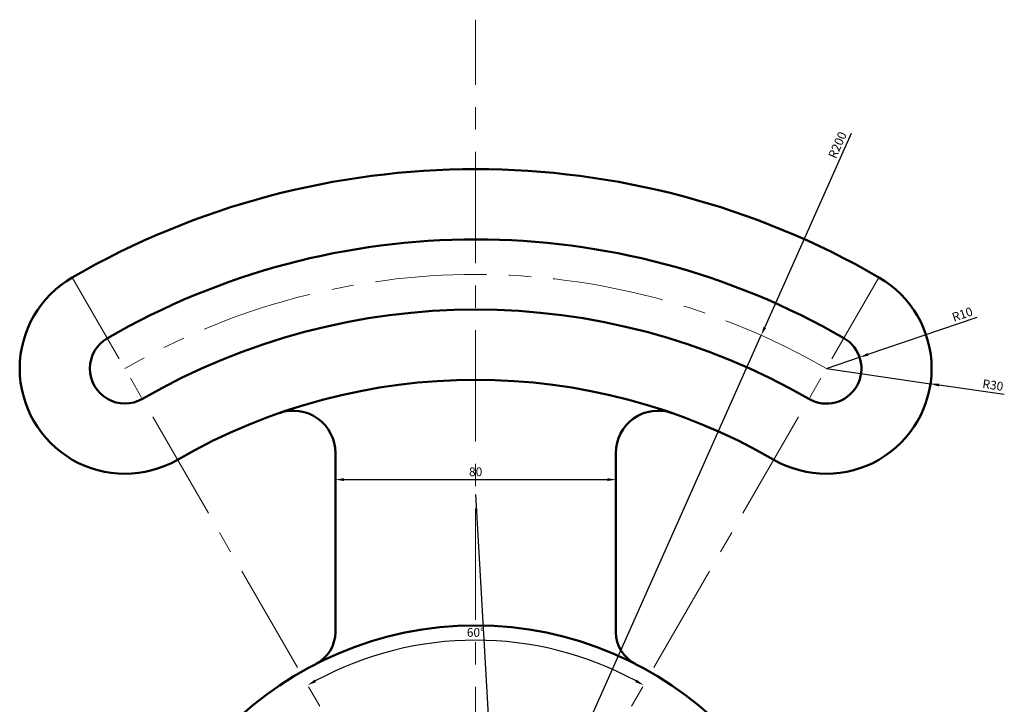
# Model space of a CAD drawing. Units: millimetres. Extents: x 107046 to 107591, y 80056 to 80641.
# Tile 3 of 3: x 107125 to 107406, y 80446 to 80641. Entities that reach past the tile are written whole.
import ezdxf

# ---------------------------------------------------------------- set-up
doc = ezdxf.new("R2010")
doc.units = ezdxf.units.MM
doc.linetypes.add('CENTER', pattern=[50.8, 31.75, -6.35, 6.35, -6.35])
for name, color, linetype, lineweight in [('M-CNTR', 1, 'CENTER', 18), ('M-DIMS', 2, 'Continuous', 25), ('M-OUTL', 7, 'Continuous', 50)]:
    doc.layers.add(name, color=color, linetype=linetype, lineweight=lineweight)
doc.styles.get("Standard").update_dxf_attribs({"font": 'arial.ttf'})
doc.dimstyles.new('ISO-25', dxfattribs={"dimtxt": 2.5, "dimasz": 2.5, "dimexe": 1.25, "dimexo": 0.625, "dimtad": 1, "dimtxsty": 'Standard', "dimcen": 2.5, "dimadec": 0, "dimazin": 0, "dimtfac": 1, "dimtmove": 0, "dimatfit": 3, "dimfxl": 1, "dimarcsym": 0})

# ---------------------------------------------------------------- blocks, each defined once
blk = doc.blocks.new('*D9')
at = {"layer": 'Defpoints', "color": 0, "transparency": 16777216}
for p in [(107295.14, 80510.33), (107215.14, 80499.73), (107295.14, 80499.73)]:
    blk.add_point(p, dxfattribs=at)
at = {"layer": 'M-DIMS', "color": 0, "lineweight": -2, "transparency": 16777216}
for p, q in [((107215.14, 80500.35), (107215.14, 80511.58)), ((107217.64, 80510.33), (107292.64, 80510.33)), ((107295.14, 80500.35), (107295.14, 80511.58))]:
    blk.add_line(p, q, dxfattribs=at)
at = {"layer": 'M-DIMS', "color": 0, "transparency": 16777216}
for points in [[(107217.64, 80510.75), (107217.64, 80509.92), (107215.14, 80510.33)], [(107292.64, 80510.75), (107292.64, 80509.92), (107295.14, 80510.33)]]:
    blk.add_solid(points, dxfattribs=at)
at = {"layer": 'M-DIMS', "color": 0, "transparency": 16777216, "insert": (107255.14, 80512.24), "char_height": 2.5, "attachment_point": 5}
blk.add_mtext('80', dxfattribs=at)
blk = doc.blocks.new('*D10')
at = {"layer": 'Defpoints', "color": 0, "transparency": 16777216}
for p in [(107364.61, 80545.19), (107355.14, 80541.99)]:
    blk.add_point(p, dxfattribs=at)
at = {"layer": 'M-DIMS', "color": 0, "lineweight": -2, "transparency": 16777216}
for p, q in [((107398.03, 80556.48), (107366.98, 80545.99)), ((107355.14, 80541.99), (107364.61, 80545.19))]:
    blk.add_line(p, q, dxfattribs=at)
at = {"layer": 'M-DIMS', "color": 0, "transparency": 16777216}
blk.add_solid([(107366.85, 80546.38), (107367.11, 80545.6), (107364.61, 80545.19)], dxfattribs=at)
at = {"layer": 'M-DIMS', "color": 0, "transparency": 16777216, "insert": (107394, 80557.13), "char_height": 2.5, "attachment_point": 5, "rotation": 18.6685}
blk.add_mtext('R10', dxfattribs=at)
blk = doc.blocks.new('*D11')
at = {"layer": 'Defpoints', "color": 0, "transparency": 16777216}
for p in [(107355.14, 80541.99), (107384.82, 80537.63)]:
    blk.add_point(p, dxfattribs=at)
at = {"layer": 'M-DIMS', "color": 0, "lineweight": -2, "transparency": 16777216}
for p, q in [((107355.14, 80541.99), (107384.82, 80537.63)), ((107405.86, 80534.54), (107387.29, 80537.27))]:
    blk.add_line(p, q, dxfattribs=at)
at = {"layer": 'M-DIMS', "color": 0, "transparency": 16777216}
blk.add_solid([(107387.35, 80537.68), (107387.23, 80536.86), (107384.82, 80537.63)], dxfattribs=at)
at = {"layer": 'M-DIMS', "color": 0, "transparency": 16777216, "insert": (107402.57, 80536.95), "char_height": 2.5, "attachment_point": 5, "rotation": 351.649}
blk.add_mtext('R30', dxfattribs=at)
blk = doc.blocks.new('*D12')
at = {"layer": 'Defpoints', "color": 0, "transparency": 16777216}
for p in [(107336.56, 80551.46), (107255.14, 80368.78)]:
    blk.add_point(p, dxfattribs=at)
at = {"layer": 'M-DIMS', "color": 0, "lineweight": -2, "transparency": 16777216}
for p, q in [((107362.18, 80608.95), (107337.58, 80553.74)), ((107255.14, 80368.78), (107336.56, 80551.46))]:
    blk.add_line(p, q, dxfattribs=at)
at = {"layer": 'M-DIMS', "color": 0, "transparency": 16777216}
blk.add_solid([(107337.2, 80553.91), (107337.96, 80553.57), (107336.56, 80551.46)], dxfattribs=at)
at = {"layer": 'M-DIMS', "color": 0, "transparency": 16777216, "insert": (107358.58, 80605.54), "char_height": 2.5, "attachment_point": 5, "rotation": 65.9766}
blk.add_mtext('R200', dxfattribs=at)
blk = doc.blocks.new('*D15')
at = {"layer": 'Defpoints', "color": 0, "transparency": 16777216}
for p in [(107255.14, 80506.08), (107277.92, 80106.73)]:
    blk.add_point(p, dxfattribs=at)
at = {"layer": 'M-DIMS', "color": 0, "lineweight": -2, "transparency": 16777216}
for p, q in [((107255.14, 80506.08), (107277.92, 80106.73)), ((107279.09, 80086.26), (107278.07, 80104.24))]:
    blk.add_line(p, q, dxfattribs=at)
at = {"layer": 'M-DIMS', "color": 0, "transparency": 16777216}
blk.add_solid([(107278.48, 80104.26), (107277.65, 80104.21), (107277.92, 80106.73)], dxfattribs=at)
at = {"layer": 'M-DIMS', "color": 0, "transparency": 16777216, "insert": (107280.73, 80090.94), "char_height": 2.5, "attachment_point": 5, "rotation": 273.2659}
blk.add_mtext('R400', dxfattribs=at)
blk = doc.blocks.new('*D18')
at = {"layer": 'Defpoints', "color": 0, "transparency": 16777216}
for p in [(107140.14, 80567.97), (107370.14, 80567.97), (107271.77, 80463.13), (107255.14, 80368.78), (107255.14, 80368.78)]:
    blk.add_point(p, dxfattribs=at)
at = {"layer": 'M-DIMS', "color": 0, "lineweight": -2, "transparency": 16777216}
blk.add_arc((107255.14, 80368.78), 95.8, 61.4952, 118.5048, dxfattribs=at)
at = {"layer": 'M-DIMS', "color": 0, "transparency": 16777216}
for points in [[(107209.62, 80452.61), (107209.21, 80453.33), (107207.24, 80451.75)], [(107301.06, 80453.33), (107300.65, 80452.61), (107303.04, 80451.75)]]:
    blk.add_solid(points, dxfattribs=at)
at = {"layer": 'M-DIMS', "color": 0, "transparency": 16777216, "insert": (107255.14, 80466.48), "char_height": 2.5, "attachment_point": 5}
blk.add_mtext('60°', dxfattribs=at)

msp = doc.modelspace()

# ---------------------------------------------------------------- linework, layer by layer
at = {"layer": 'M-CNTR'}
for p, q in [((107255.136, 80368.784), (107255.136, 80641.38)), ((107255.136, 80368.784), (107140.136, 80567.97)), ((107255.136, 80368.784), (107370.136, 80567.97)), ((107318.961, 80558.326), (107318.961, 80558.326))]:
    msp.add_line(p, q, dxfattribs=at)
msp.add_arc((107255.136, 80368.784), 200, 60, 120, dxfattribs=at)
at = {"layer": 'M-OUTL'}
for p, q in [((107215.136, 80502.097), (107215.136, 80517.982)), ((107215.136, 80517.982), (107215.136, 80466.904)), ((107295.136, 80466.904), (107295.136, 80517.982))]:
    msp.add_line(p, q, dxfattribs=at)
msp.add_circle((107255.136, 80368.784), 100, dxfattribs=at)
for centre, radius, start, end in [((107255.136, 80368.784), 230, 60, 120), ((107255.136, 80368.784), 210, 60, 120), ((107155.136, 80541.989), 30, 119.99997, 300.00003), ((107355.136, 80541.989), 30, 239.99997, 60.00003), ((107255.136, 80368.784), 190, 60, 120), ((107155.136, 80541.989), 10, 120, 300), ((107355.136, 80541.989), 10, 240, 60), ((107255.136, 80368.784), 170, 60, 120), ((107203.136, 80517.982), 12, 0, 109.215), ((107307.136, 80517.982), 12, 70.785, 180), ((107204.907, 80466.904), 10.229, 297.10869, 0), ((107305.366, 80466.904), 10.229, 180, 242.89131)]:
    msp.add_arc(centre, radius, start, end, dxfattribs=at)

# ---------------------------------------------------------------- dimensions: what is measured, and where the dimension line sits
at = {"layer": 'M-DIMS'}
for center, mpoint, picture, middle in [((107255.136, 80368.784), (107336.558, 80551.46), '*D12', (107360.32, 80604.77)), ((107355.136, 80541.989), (107364.61, 80545.19), '*D10', (107394.608, 80555.325)), ((107355.136, 80541.989), (107384.818, 80537.632), '*D11', (107402.295, 80535.066)), ((107255.136, 80506.082), (107277.924, 80106.732), '*D15', (107278.831, 80090.833))]:
    dim = msp.add_radius_dim(center=center, mpoint=mpoint, dimstyle='ISO-25', override={"dimclrd": 0, "dimclre": 0, "dimclrt": 0}, dxfattribs=at)
    dim.commit()
    dim.dimension.update_dxf_attribs({"geometry": picture, "text_midpoint": middle, "dimtype": 164})
dim = msp.add_angular_dim_2l(base=(107271.772, 80463.128), line1=((107255.136, 80368.784), (107370.136, 80567.97)), line2=((107255.136, 80368.784), (107140.136, 80567.97)), dimstyle='ISO-25', override={"dimclrd": 0, "dimclre": 0, "dimclrt": 0}, dxfattribs=at)
dim.commit()
dim.dimension.update_dxf_attribs({"geometry": '*D18', "text_midpoint": (107255.136, 80466.485)})
dim = msp.add_linear_dim(base=(107295.136, 80510.335), p1=(107215.136, 80499.727), p2=(107295.136, 80499.727), dimstyle='ISO-25', override={"dimclrd": 0, "dimclre": 0, "dimclrt": 0}, dxfattribs=at)
dim.commit()
dim.dimension.update_dxf_attribs({"geometry": '*D9', "text_midpoint": (107255.136, 80512.236)})

doc.saveas('drawing.dxf')
